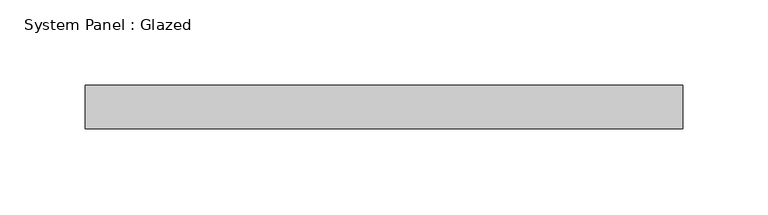
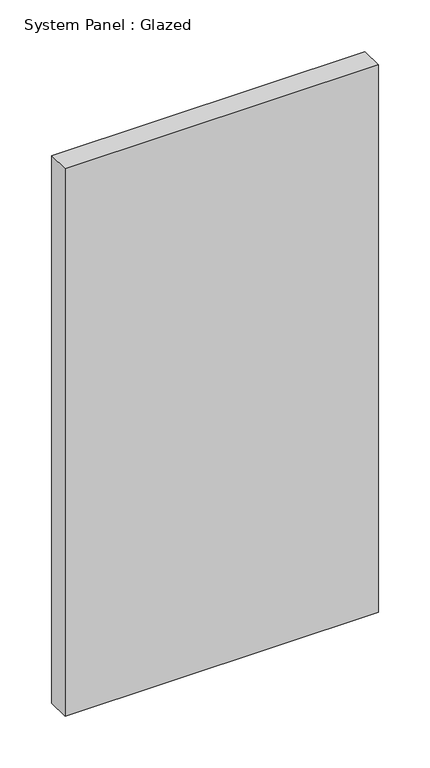
"""IFC4 building model written with IfcOpenShell, lengths in millimetres: plate geometry, System Panel : Glazed."""

from ifc_helpers import new_model, si_unit, origin, origin_with_axes, place, context, project, spatial, polyline, outline, extrude, source, transform, mapped, element, save


def system_panel_glazed_5f4e04c5(model_context):
    return source(origin(), model_context, "Body", "SweptSolid", [
        extrude(outline(polyline([(174.625, 19.05), (-174.625, 19.05), (-174.625, 44.45), (174.625, 44.45), (174.625, 19.05)])), origin_with_axes(), (0.0, 0.0, 1.0), 644.585164),
    ])


if __name__ == "__main__":
    model = new_model("IFC4")
    model_context = context("Model", 3, world=origin())
    ifc_project = project(units=[si_unit("LENGTHUNIT", "METRE", prefix="MILLI")], contexts=[model_context])
    site = spatial("IfcSite", under=ifc_project)
    building = spatial("IfcBuilding", under=site)
    placement = place(None, origin())
    system_panel_glazed_shape = system_panel_glazed_5f4e04c5(model_context)
    element("IfcPlate", 1, ObjectType="System Panel : Glazed", at=placement, inside=building, context=model_context, shape_type="MappedRepresentation", body=[
        mapped(system_panel_glazed_shape, transform((0.0, 0.0, 0.0), x_axis=(1.0, 0.0, 0.0), y_axis=(0.0, 1.0, 0.0), z_axis=(0.0, 0.0, 1.0))),
    ])
    save(model, "model.ifc")

# Revit data of these elements
# Type "System Panel : Glazed"
#   Construction Type Id = "GSP4R"
#   Analytic Construction = "1/8 in Pilkington single glazing"
#   Visual Light Transmittance = 0.9
#   Solar Heat Gain Coefficient = 0.86
#   Heat Transfer Coefficient (U) = 1.18115 BTU/(h·ft²·°F)
#   Define Thermal Properties by = 1
# Element 1 (IfcPlate, "System Panel : Glazed")
#   Materials on its faces: "Glass"
# Materials
#   "Glass": class "Glass", colour RGB 0 128 192, transparency 0.75, Description = "Soda Lime Glass", Cost = 0
